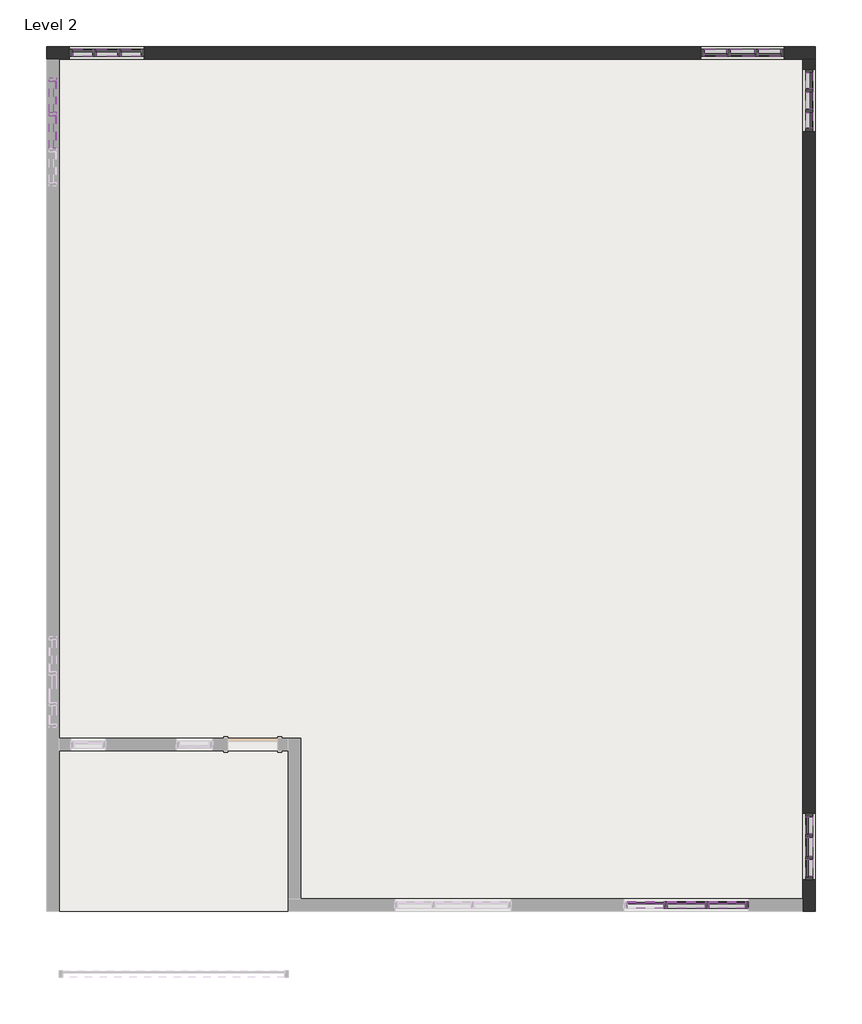
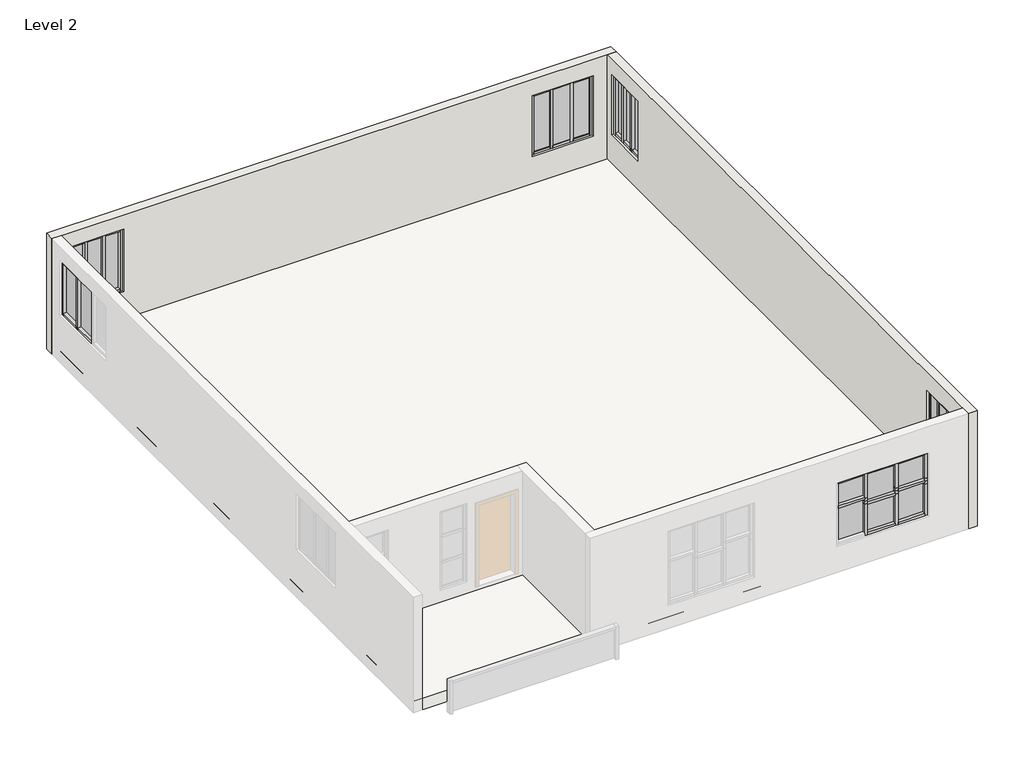
# One storey, part 2 of 2: 65 members, 20 plates, 2 walls, 1 roof.
"""IFC4 building model written with IfcOpenShell, lengths in millimetres."""

from ifc_helpers import new_model, si_unit, frame, origin, place, context, project, spatial, polyline, outline, extrude, faceted_brep, transform, mapped, element, save
from components import member_dc106669, member_bc7dbe04, member_b955a9e9, member_c33c434a, member_5ad95953, member_ff1b7d8f, member_c71c3647, member_d485efb4, member_6c34f49c, member_3060f3e2, member_dfbe775a, member_db0015e1, member_7096a90e, member_843225dc, member_fad113ab, member_ea29af33, member_6f432376, member_04a79ac1, member_a400357f, member_b1615173, member_de6f3820, member_f53dc333, member_00d00b53, member_c7c5a8a0, member_d6240b74, member_2ee2964b, member_655cfd9b, member_3d7cb871, member_3cc62806, member_2ad165f7, system_panel_glazed_811a1c5c, system_panel_glazed_f11b7ff6, system_panel_glazed_c33e710a, system_panel_glazed_37470fb4, system_panel_glazed_1aec69dd, system_panel_glazed_f4403250, system_panel_glazed_a7448bf8, system_panel_glazed_01fedee4, system_panel_glazed_02e859a2, system_panel_glazed_cd5540fc, system_panel_glazed_1b56a55a, system_panel_glazed_4819e94b, system_panel_glazed_cfa4a589, system_panel_glazed_093ce7df, system_panel_glazed_0a1fe405, system_panel_glazed_81358e4c

model = new_model("IFC4")

# Units and contexts
model_context = context("Model", 3, world=origin())
ifc_project = project(units=[si_unit("LENGTHUNIT", "METRE", prefix="MILLI")], contexts=[model_context])

# Site, building, storey
site = spatial("IfcSite", under=ifc_project)
building = spatial("IfcBuilding", under=site)
storey = spatial("IfcBuildingStorey", under=building, Name="Level 2", Elevation=3048.0)

# Members
placement = place(None, origin())
member_shape = member_dc106669(model_context)
element("IfcMember", 1, ObjectType="Rectangular Mullion : 2.5\" x 5\" rectangular", at=placement, inside=storey, context=model_context, shape_type="MappedRepresentation", body=[
    mapped(member_shape, transform((-8840.6597681, 1450.4660078, 5670.8139768), x_axis=(0.0, 0.0, 1.0), y_axis=(0.0, 1.0, 0.0), z_axis=(-1.0, 0.0, 0.0))),
])
element("IfcMember", 2, ObjectType="Rectangular Mullion : 2.5\" x 5\" rectangular", at=placement, inside=storey, context=model_context, shape_type="MappedRepresentation", body=[
    mapped(member_shape, transform((-9824.9097681, 1450.4660078, 5670.8139768), x_axis=(0.0, 0.0, 1.0), y_axis=(0.0, 1.0, 0.0), z_axis=(-1.0, 0.0, 0.0))),
])
member_2_shape = member_bc7dbe04(model_context)
element("IfcMember", 3, ObjectType="Rectangular Mullion : 2.5\" x 5\" rectangular", at=placement, inside=storey, context=model_context, shape_type="MappedRepresentation", body=[
    mapped(member_2_shape, transform((-9348.6597681, 1450.4660078, 5670.8139768), x_axis=(0.0, 0.0, 1.0), y_axis=(0.0, 1.0, 0.0), z_axis=(-1.0, 0.0, 0.0))),
])
element("IfcMember", 4, ObjectType="Rectangular Mullion : 2.5\" x 5\" rectangular", at=placement, inside=storey, context=model_context, shape_type="MappedRepresentation", body=[
    mapped(member_2_shape, transform((-8904.1597681, 1450.4660078, 4071.2518782), x_axis=(0.0, 0.0, -1.0), y_axis=(0.0, 1.0, 0.0), z_axis=(1.0, 0.0, 0.0))),
])
element("IfcMember", 5, ObjectType="Rectangular Mullion : 2.5\" x 5\" rectangular", at=placement, inside=storey, context=model_context, shape_type="MappedRepresentation", body=[
    mapped(member_shape, transform((-9412.1597681, 1450.4660078, 4071.2518782), x_axis=(0.0, 0.0, -1.0), y_axis=(0.0, 1.0, 0.0), z_axis=(1.0, 0.0, 0.0))),
])
element("IfcMember", 6, ObjectType="Rectangular Mullion : 2.5\" x 5\" rectangular", at=placement, inside=storey, context=model_context, shape_type="MappedRepresentation", body=[
    mapped(member_shape, transform((-8427.9097681, 1450.4660078, 4071.2518782), x_axis=(0.0, 0.0, -1.0), y_axis=(0.0, 1.0, 0.0), z_axis=(1.0, 0.0, 0.0))),
])
member_3_shape = member_b955a9e9(model_context)
element("IfcMember", 7, ObjectType="Rectangular Mullion : 2.5\" x 5\" rectangular", at=placement, inside=storey, context=model_context, shape_type="MappedRepresentation", body=[
    mapped(member_3_shape, transform((-9805.8597681, -14132.4339922, 5397.3589008), x_axis=(0.0, 0.0, 1.0), y_axis=(0.0, -1.0, 0.0), z_axis=(1.0, 0.0, 0.0))),
])
member_4_shape = member_c33c434a(model_context)
element("IfcMember", 8, ObjectType="Rectangular Mullion : 2.5\" x 5\" rectangular", at=placement, inside=storey, context=model_context, shape_type="MappedRepresentation", body=[
    mapped(member_4_shape, transform((-10567.8597681, -14132.4339922, 5397.3589008), x_axis=(0.0, 0.0, 1.0), y_axis=(0.0, -1.0, 0.0), z_axis=(1.0, 0.0, 0.0))),
])
element("IfcMember", 9, ObjectType="Rectangular Mullion : 2.5\" x 5\" rectangular", at=placement, inside=storey, context=model_context, shape_type="MappedRepresentation", body=[
    mapped(member_4_shape, transform((-9075.6097681, -14132.4339922, 5397.3589008), x_axis=(0.0, 0.0, 1.0), y_axis=(0.0, -1.0, 0.0), z_axis=(1.0, 0.0, 0.0))),
])
element("IfcMember", 10, ObjectType="Rectangular Mullion : 2.5\" x 5\" rectangular", at=placement, inside=storey, context=model_context, shape_type="MappedRepresentation", body=[
    mapped(member_4_shape, transform((-9742.3597681, -14132.4339922, 3732.481147), x_axis=(0.0, 0.0, -1.0), y_axis=(0.0, -1.0, 0.0), z_axis=(-1.0, 0.0, 0.0))),
])
element("IfcMember", 11, ObjectType="Rectangular Mullion : 2.5\" x 5\" rectangular", at=placement, inside=storey, context=model_context, shape_type="MappedRepresentation", body=[
    mapped(member_3_shape, transform((-10504.3597681, -14132.4339922, 3732.481147), x_axis=(0.0, 0.0, -1.0), y_axis=(0.0, -1.0, 0.0), z_axis=(-1.0, 0.0, 0.0))),
])
member_5_shape = member_5ad95953(model_context)
element("IfcMember", 12, ObjectType="Rectangular Mullion : 2.5\" x 5\" rectangular", at=placement, inside=storey, context=model_context, shape_type="MappedRepresentation", body=[
    mapped(member_5_shape, transform((-7907.2097681, -13300.5839922, 5612.7165878), x_axis=(0.0, 0.0, 1.0), y_axis=(1.0, 0.0, 0.0), z_axis=(0.0, 1.0, 0.0))),
])
element("IfcMember", 13, ObjectType="Rectangular Mullion : 2.5\" x 5\" rectangular", at=placement, inside=storey, context=model_context, shape_type="MappedRepresentation", body=[
    mapped(member_5_shape, transform((-7907.2097681, -12519.5339922, 5612.7165878), x_axis=(0.0, 0.0, 1.0), y_axis=(1.0, 0.0, 0.0), z_axis=(0.0, 1.0, 0.0))),
])
member_6_shape = member_ff1b7d8f(model_context)
element("IfcMember", 14, ObjectType="Rectangular Mullion : 2.5\" x 5\" rectangular", at=placement, inside=storey, context=model_context, shape_type="MappedRepresentation", body=[
    mapped(member_6_shape, transform((-7907.2097681, -12894.1839922, 5612.7165878), x_axis=(0.0, 0.0, 1.0), y_axis=(1.0, 0.0, 0.0), z_axis=(0.0, 1.0, 0.0))),
])
member_7_shape = member_c71c3647(model_context)
element("IfcMember", 15, ObjectType="Rectangular Mullion : 2.5\" x 5\" rectangular", at=placement, inside=storey, context=model_context, shape_type="MappedRepresentation", body=[
    mapped(member_7_shape, transform((-7907.2097681, -12862.4339922, 4117.147182), x_axis=(0.0, 1.0, 0.0), y_axis=(1.0, 0.0, 0.0), z_axis=(0.0, 0.0, -1.0))),
])
element("IfcMember", 16, ObjectType="Rectangular Mullion : 2.5\" x 5\" rectangular", at=placement, inside=storey, context=model_context, shape_type="MappedRepresentation", body=[
    mapped(member_7_shape, transform((-7907.2097681, -13268.8339922, 4117.147182), x_axis=(0.0, 1.0, 0.0), y_axis=(1.0, 0.0, 0.0), z_axis=(0.0, 0.0, -1.0))),
])
element("IfcMember", 17, ObjectType="Rectangular Mullion : 2.5\" x 5\" rectangular", at=placement, inside=storey, context=model_context, shape_type="MappedRepresentation", body=[
    mapped(member_5_shape, transform((-7907.2097681, -12830.6839922, 4117.147182), x_axis=(0.0, 0.0, -1.0), y_axis=(1.0, 0.0, 0.0), z_axis=(0.0, -1.0, 0.0))),
])
element("IfcMember", 18, ObjectType="Rectangular Mullion : 2.5\" x 5\" rectangular", at=placement, inside=storey, context=model_context, shape_type="MappedRepresentation", body=[
    mapped(member_5_shape, transform((-7907.2097681, -13611.7339922, 4117.147182), x_axis=(0.0, 0.0, -1.0), y_axis=(1.0, 0.0, 0.0), z_axis=(0.0, -1.0, 0.0))),
])
element("IfcMember", 19, ObjectType="Rectangular Mullion : 2.5\" x 5\" rectangular", at=placement, inside=storey, context=model_context, shape_type="MappedRepresentation", body=[
    mapped(member_6_shape, transform((-7907.2097681, -13237.0839922, 4117.147182), x_axis=(0.0, 0.0, -1.0), y_axis=(1.0, 0.0, 0.0), z_axis=(0.0, -1.0, 0.0))),
])
member_8_shape = member_d485efb4(model_context)
element("IfcMember", 20, ObjectType="Rectangular Mullion : 2.5\" x 5\" rectangular", at=placement, inside=storey, context=model_context, shape_type="MappedRepresentation", body=[
    mapped(member_8_shape, transform((-7907.2097681, -12456.0339922, 4117.147182), x_axis=(0.0, 1.0, 0.0), y_axis=(1.0, 0.0, 0.0), z_axis=(0.0, 0.0, -1.0))),
])
element("IfcMember", 21, ObjectType="Rectangular Mullion : 2.5\" x 5\" rectangular", at=placement, inside=storey, context=model_context, shape_type="MappedRepresentation", body=[
    mapped(member_8_shape, transform((-7907.2097681, -13675.2339922, 5612.7165878), x_axis=(0.0, -1.0, 0.0), y_axis=(1.0, 0.0, 0.0), z_axis=(0.0, 0.0, 1.0))),
])
member_9_shape = member_6c34f49c(model_context)
element("IfcMember", 22, ObjectType="Rectangular Mullion : 2.5\" x 5\" rectangular", at=placement, inside=storey, context=model_context, shape_type="MappedRepresentation", body=[
    mapped(member_9_shape, transform((-7907.2097681, 796.4160078, 5681.6996077), x_axis=(0.0, 0.0, 1.0), y_axis=(-1.0, 0.0, 0.0), z_axis=(0.0, -1.0, 0.0))),
])
element("IfcMember", 23, ObjectType="Rectangular Mullion : 2.5\" x 5\" rectangular", at=placement, inside=storey, context=model_context, shape_type="MappedRepresentation", body=[
    mapped(member_9_shape, transform((-7907.2097681, 66.1660078, 5681.6996077), x_axis=(0.0, 0.0, 1.0), y_axis=(-1.0, 0.0, 0.0), z_axis=(0.0, -1.0, 0.0))),
])
member_10_shape = member_3060f3e2(model_context)
element("IfcMember", 24, ObjectType="Rectangular Mullion : 2.5\" x 5\" rectangular", at=placement, inside=storey, context=model_context, shape_type="MappedRepresentation", body=[
    mapped(member_10_shape, transform((-7907.2097681, 415.4160078, 5681.6996077), x_axis=(0.0, 0.0, 1.0), y_axis=(-1.0, 0.0, 0.0), z_axis=(0.0, -1.0, 0.0))),
])
member_11_shape = member_dfbe775a(model_context)
element("IfcMember", 25, ObjectType="Rectangular Mullion : 2.5\" x 5\" rectangular", at=placement, inside=storey, context=model_context, shape_type="MappedRepresentation", body=[
    mapped(member_11_shape, transform((-7907.2097681, 383.6660078, 4107.4707945), x_axis=(0.0, -1.0, 0.0), y_axis=(-1.0, 0.0, 0.0), z_axis=(0.0, 0.0, -1.0))),
])
element("IfcMember", 26, ObjectType="Rectangular Mullion : 2.5\" x 5\" rectangular", at=placement, inside=storey, context=model_context, shape_type="MappedRepresentation", body=[
    mapped(member_11_shape, transform((-7907.2097681, 764.6660078, 4107.4707945), x_axis=(0.0, -1.0, 0.0), y_axis=(-1.0, 0.0, 0.0), z_axis=(0.0, 0.0, -1.0))),
])
element("IfcMember", 27, ObjectType="Rectangular Mullion : 2.5\" x 5\" rectangular", at=placement, inside=storey, context=model_context, shape_type="MappedRepresentation", body=[
    mapped(member_10_shape, transform((-7907.2097681, 732.9160078, 4107.4707945), x_axis=(0.0, 0.0, -1.0), y_axis=(-1.0, 0.0, 0.0), z_axis=(0.0, 1.0, 0.0))),
])
element("IfcMember", 28, ObjectType="Rectangular Mullion : 2.5\" x 5\" rectangular", at=placement, inside=storey, context=model_context, shape_type="MappedRepresentation", body=[
    mapped(member_9_shape, transform((-7907.2097681, 351.9160078, 4107.4707945), x_axis=(0.0, 0.0, -1.0), y_axis=(-1.0, 0.0, 0.0), z_axis=(0.0, 1.0, 0.0))),
])
element("IfcMember", 29, ObjectType="Rectangular Mullion : 2.5\" x 5\" rectangular", at=placement, inside=storey, context=model_context, shape_type="MappedRepresentation", body=[
    mapped(member_9_shape, transform((-7907.2097681, 1082.1660078, 4107.4707945), x_axis=(0.0, 0.0, -1.0), y_axis=(-1.0, 0.0, 0.0), z_axis=(0.0, 1.0, 0.0))),
])
member_12_shape = member_db0015e1(model_context)
element("IfcMember", 30, ObjectType="Rectangular Mullion : 2.5\" x 5\" rectangular", at=placement, inside=storey, context=model_context, shape_type="MappedRepresentation", body=[
    mapped(member_12_shape, transform((-7907.2097681, 1145.6660078, 5681.6996077), x_axis=(0.0, 1.0, 0.0), y_axis=(-1.0, 0.0, 0.0), z_axis=(0.0, 0.0, 1.0))),
])
element("IfcMember", 31, ObjectType="Rectangular Mullion : 2.5\" x 5\" rectangular", at=placement, inside=storey, context=model_context, shape_type="MappedRepresentation", body=[
    mapped(member_12_shape, transform((-7907.2097681, 2.6660078, 4107.4707945), x_axis=(0.0, -1.0, 0.0), y_axis=(-1.0, 0.0, 0.0), z_axis=(0.0, 0.0, -1.0))),
])
member_13_shape = member_7096a90e(model_context)
element("IfcMember", 32, ObjectType="Rectangular Mullion : 2.5\" x 5\" rectangular", at=placement, inside=storey, context=model_context, shape_type="MappedRepresentation", body=[
    mapped(member_13_shape, transform((-20550.0597681, 1450.4660078, 5713.3390555), x_axis=(0.0, 0.0, 1.0), y_axis=(0.0, -1.0, 0.0), z_axis=(1.0, 0.0, 0.0))),
])
member_14_shape = member_843225dc(model_context)
element("IfcMember", 33, ObjectType="Rectangular Mullion : 2.5\" x 5\" rectangular", at=placement, inside=storey, context=model_context, shape_type="MappedRepresentation", body=[
    mapped(member_14_shape, transform((-21007.2597681, 1450.4660078, 5713.3390555), x_axis=(0.0, 0.0, 1.0), y_axis=(0.0, -1.0, 0.0), z_axis=(1.0, 0.0, 0.0))),
])
element("IfcMember", 34, ObjectType="Rectangular Mullion : 2.5\" x 5\" rectangular", at=placement, inside=storey, context=model_context, shape_type="MappedRepresentation", body=[
    mapped(member_14_shape, transform((-20124.6097681, 1450.4660078, 5713.3390555), x_axis=(0.0, 0.0, 1.0), y_axis=(0.0, -1.0, 0.0), z_axis=(1.0, 0.0, 0.0))),
])
member_15_shape = member_fad113ab(model_context)
element("IfcMember", 35, ObjectType="Rectangular Mullion : 2.5\" x 5\" rectangular", at=placement, inside=storey, context=model_context, shape_type="MappedRepresentation", body=[
    mapped(member_15_shape, transform((-20518.3097681, 1450.4660078, 4066.3851852), x_axis=(1.0, 0.0, 0.0), y_axis=(0.0, -1.0, 0.0), z_axis=(0.0, 0.0, -1.0))),
])
element("IfcMember", 36, ObjectType="Rectangular Mullion : 2.5\" x 5\" rectangular", at=placement, inside=storey, context=model_context, shape_type="MappedRepresentation", body=[
    mapped(member_15_shape, transform((-20975.5097681, 1450.4660078, 4066.3851852), x_axis=(1.0, 0.0, 0.0), y_axis=(0.0, -1.0, 0.0), z_axis=(0.0, 0.0, -1.0))),
])
element("IfcMember", 37, ObjectType="Rectangular Mullion : 2.5\" x 5\" rectangular", at=placement, inside=storey, context=model_context, shape_type="MappedRepresentation", body=[
    mapped(member_13_shape, transform((-20943.7597681, 1450.4660078, 4066.3851852), x_axis=(0.0, 0.0, -1.0), y_axis=(0.0, -1.0, 0.0), z_axis=(-1.0, 0.0, 0.0))),
])
element("IfcMember", 38, ObjectType="Rectangular Mullion : 2.5\" x 5\" rectangular", at=placement, inside=storey, context=model_context, shape_type="MappedRepresentation", body=[
    mapped(member_14_shape, transform((-20486.5597681, 1450.4660078, 4066.3851852), x_axis=(0.0, 0.0, -1.0), y_axis=(0.0, -1.0, 0.0), z_axis=(-1.0, 0.0, 0.0))),
])
element("IfcMember", 39, ObjectType="Rectangular Mullion : 2.5\" x 5\" rectangular", at=placement, inside=storey, context=model_context, shape_type="MappedRepresentation", body=[
    mapped(member_14_shape, transform((-21369.2097681, 1450.4660078, 4066.3851852), x_axis=(0.0, 0.0, -1.0), y_axis=(0.0, -1.0, 0.0), z_axis=(-1.0, 0.0, 0.0))),
])
member_16_shape = member_ea29af33(model_context)
element("IfcMember", 40, ObjectType="Rectangular Mullion : 2.5\" x 5\" rectangular", at=placement, inside=storey, context=model_context, shape_type="MappedRepresentation", body=[
    mapped(member_16_shape, transform((-21432.7097681, 1450.4660078, 5713.3390555), x_axis=(-1.0, 0.0, 0.0), y_axis=(0.0, -1.0, 0.0), z_axis=(0.0, 0.0, 1.0))),
])
element("IfcMember", 41, ObjectType="Rectangular Mullion : 2.5\" x 5\" rectangular", at=placement, inside=storey, context=model_context, shape_type="MappedRepresentation", body=[
    mapped(member_16_shape, transform((-20061.1097681, 1450.4660078, 4066.3851852), x_axis=(1.0, 0.0, 0.0), y_axis=(0.0, -1.0, 0.0), z_axis=(0.0, 0.0, -1.0))),
])
member_17_shape = member_6f432376(model_context)
element("IfcMember", 42, ObjectType="Rectangular Mullion : 2.5\" x 5\" rectangular", at=placement, inside=storey, context=model_context, shape_type="MappedRepresentation", body=[
    mapped(member_17_shape, transform((-21737.5097681, 364.6160078, 5718.9037492), x_axis=(0.0, 0.0, 1.0), y_axis=(-1.0, 0.0, 0.0), z_axis=(0.0, -1.0, 0.0))),
])
member_18_shape = member_04a79ac1(model_context)
element("IfcMember", 43, ObjectType="Rectangular Mullion : 2.5\" x 5\" rectangular", at=placement, inside=storey, context=model_context, shape_type="MappedRepresentation", body=[
    mapped(member_18_shape, transform((-21737.5097681, 332.8660078, 4287.8866443), x_axis=(0.0, -1.0, 0.0), y_axis=(-1.0, 0.0, 0.0), z_axis=(0.0, 0.0, -1.0))),
])
element("IfcMember", 44, ObjectType="Rectangular Mullion : 2.5\" x 5\" rectangular", at=placement, inside=storey, context=model_context, shape_type="MappedRepresentation", body=[
    mapped(member_17_shape, transform((-21737.5097681, 929.7660078, 4287.8866443), x_axis=(0.0, 0.0, -1.0), y_axis=(-1.0, 0.0, 0.0), z_axis=(0.0, 1.0, 0.0))),
])
member_19_shape = member_a400357f(model_context)
element("IfcMember", 45, ObjectType="Rectangular Mullion : 2.5\" x 5\" rectangular", at=placement, inside=storey, context=model_context, shape_type="MappedRepresentation", body=[
    mapped(member_19_shape, transform((-21737.5097681, 301.1160078, 4287.8866443), x_axis=(0.0, 0.0, -1.0), y_axis=(-1.0, 0.0, 0.0), z_axis=(0.0, 1.0, 0.0))),
])
member_20_shape = member_b1615173(model_context)
element("IfcMember", 46, ObjectType="Rectangular Mullion : 2.5\" x 5\" rectangular", at=placement, inside=storey, context=model_context, shape_type="MappedRepresentation", body=[
    mapped(member_20_shape, transform((-21737.5097681, 993.2660078, 5718.9037492), x_axis=(0.0, 1.0, 0.0), y_axis=(-1.0, 0.0, 0.0), z_axis=(0.0, 0.0, 1.0))),
])
member_21_shape = member_de6f3820(model_context)
element("IfcMember", 47, ObjectType="Rectangular Mullion : 2.5\" x 5\" rectangular", at=placement, inside=storey, context=model_context, shape_type="MappedRepresentation", body=[
    mapped(member_21_shape, transform((-9380.4097681, 1450.4660078, 4071.2518782), x_axis=(-1.0, 0.0, 0.0), y_axis=(0.0, 1.0, 0.0), z_axis=(0.0, 0.0, -1.0))),
])
element("IfcMember", 48, ObjectType="Rectangular Mullion : 2.5\" x 5\" rectangular", at=placement, inside=storey, context=model_context, shape_type="MappedRepresentation", body=[
    mapped(member_21_shape, transform((-8872.4097681, 1450.4660078, 4071.2518782), x_axis=(-1.0, 0.0, 0.0), y_axis=(0.0, 1.0, 0.0), z_axis=(0.0, 0.0, -1.0))),
])
member_22_shape = member_f53dc333(model_context)
element("IfcMember", 49, ObjectType="Rectangular Mullion : 2.5\" x 5\" rectangular", at=placement, inside=storey, context=model_context, shape_type="MappedRepresentation", body=[
    mapped(member_22_shape, transform((-9888.4097681, 1450.4660078, 4071.2518782), x_axis=(-1.0, 0.0, 0.0), y_axis=(0.0, 1.0, 0.0), z_axis=(0.0, 0.0, -1.0))),
])
element("IfcMember", 50, ObjectType="Rectangular Mullion : 2.5\" x 5\" rectangular", at=placement, inside=storey, context=model_context, shape_type="MappedRepresentation", body=[
    mapped(member_22_shape, transform((-8364.4097681, 1450.4660078, 5670.8139768), x_axis=(1.0, 0.0, 0.0), y_axis=(0.0, 1.0, 0.0), z_axis=(0.0, 0.0, 1.0))),
])
member_23_shape = member_00d00b53(model_context)
element("IfcMember", 51, ObjectType="Rectangular Mullion : 2.5\" x 5\" rectangular", at=placement, inside=storey, context=model_context, shape_type="MappedRepresentation", body=[
    mapped(member_23_shape, transform((-9774.1097681, -14132.4339922, 4641.1200239), x_axis=(1.0, 0.0, 0.0), y_axis=(0.0, -1.0, 0.0), z_axis=(0.0, 0.0, -1.0))),
])
element("IfcMember", 52, ObjectType="Rectangular Mullion : 2.5\" x 5\" rectangular", at=placement, inside=storey, context=model_context, shape_type="MappedRepresentation", body=[
    mapped(member_23_shape, transform((-10536.1097681, -14132.4339922, 4564.9200239), x_axis=(1.0, 0.0, 0.0), y_axis=(0.0, -1.0, 0.0), z_axis=(0.0, 0.0, -1.0))),
])
element("IfcMember", 53, ObjectType="Rectangular Mullion : 2.5\" x 5\" rectangular", at=placement, inside=storey, context=model_context, shape_type="MappedRepresentation", body=[
    mapped(member_23_shape, transform((-9774.1097681, -14132.4339922, 4564.9200239), x_axis=(1.0, 0.0, 0.0), y_axis=(0.0, -1.0, 0.0), z_axis=(0.0, 0.0, -1.0))),
])
member_24_shape = member_c7c5a8a0(model_context)
element("IfcMember", 54, ObjectType="Rectangular Mullion : 2.5\" x 5\" rectangular", at=placement, inside=storey, context=model_context, shape_type="MappedRepresentation", body=[
    mapped(member_24_shape, transform((-9805.8597681, -14132.4339922, 4564.9200239), x_axis=(0.0, 0.0, 1.0), y_axis=(0.0, -1.0, 0.0), z_axis=(1.0, 0.0, 0.0))),
])
element("IfcMember", 55, ObjectType="Rectangular Mullion : 2.5\" x 5\" rectangular", at=placement, inside=storey, context=model_context, shape_type="MappedRepresentation", body=[
    mapped(member_23_shape, transform((-10536.1097681, -14132.4339922, 4641.1200239), x_axis=(1.0, 0.0, 0.0), y_axis=(0.0, -1.0, 0.0), z_axis=(0.0, 0.0, -1.0))),
])
member_25_shape = member_d6240b74(model_context)
element("IfcMember", 56, ObjectType="Rectangular Mullion : 2.5\" x 5\" rectangular", at=placement, inside=storey, context=model_context, shape_type="MappedRepresentation", body=[
    mapped(member_25_shape, transform((-9774.1097681, -14132.4339922, 4717.3200239), x_axis=(1.0, 0.0, 0.0), y_axis=(0.0, -1.0, 0.0), z_axis=(0.0, 0.0, -1.0))),
])
element("IfcMember", 57, ObjectType="Rectangular Mullion : 2.5\" x 5\" rectangular", at=placement, inside=storey, context=model_context, shape_type="MappedRepresentation", body=[
    mapped(member_25_shape, transform((-10536.1097681, -14132.4339922, 4717.3200239), x_axis=(1.0, 0.0, 0.0), y_axis=(0.0, -1.0, 0.0), z_axis=(0.0, 0.0, -1.0))),
])
member_26_shape = member_2ee2964b(model_context)
element("IfcMember", 58, ObjectType="Rectangular Mullion : 2.5\" x 5\" rectangular", at=placement, inside=storey, context=model_context, shape_type="MappedRepresentation", body=[
    mapped(member_26_shape, transform((-10567.8597681, -14132.4339922, 4717.3200239), x_axis=(0.0, 0.0, 1.0), y_axis=(0.0, -1.0, 0.0), z_axis=(1.0, 0.0, 0.0))),
])
element("IfcMember", 59, ObjectType="Rectangular Mullion : 2.5\" x 5\" rectangular", at=placement, inside=storey, context=model_context, shape_type="MappedRepresentation", body=[
    mapped(member_26_shape, transform((-9075.6097681, -14132.4339922, 4641.1200239), x_axis=(0.0, 0.0, 1.0), y_axis=(0.0, -1.0, 0.0), z_axis=(1.0, 0.0, 0.0))),
])
member_27_shape = member_655cfd9b(model_context)
element("IfcMember", 60, ObjectType="Rectangular Mullion : 2.5\" x 5\" rectangular", at=placement, inside=storey, context=model_context, shape_type="MappedRepresentation", body=[
    mapped(member_27_shape, transform((-9774.1097681, -14132.4339922, 3732.481147), x_axis=(1.0, 0.0, 0.0), y_axis=(0.0, -1.0, 0.0), z_axis=(0.0, 0.0, -1.0))),
])
element("IfcMember", 61, ObjectType="Rectangular Mullion : 2.5\" x 5\" rectangular", at=placement, inside=storey, context=model_context, shape_type="MappedRepresentation", body=[
    mapped(member_27_shape, transform((-10536.1097681, -14132.4339922, 3732.481147), x_axis=(1.0, 0.0, 0.0), y_axis=(0.0, -1.0, 0.0), z_axis=(0.0, 0.0, -1.0))),
])
member_28_shape = member_3d7cb871(model_context)
element("IfcMember", 62, ObjectType="Rectangular Mullion : 2.5\" x 5\" rectangular", at=placement, inside=storey, context=model_context, shape_type="MappedRepresentation", body=[
    mapped(member_28_shape, transform((-9012.1097681, -14132.4339922, 4641.1200239), x_axis=(1.0, 0.0, 0.0), y_axis=(0.0, -1.0, 0.0), z_axis=(0.0, 0.0, -1.0))),
])
member_29_shape = member_3cc62806(model_context)
element("IfcMember", 63, ObjectType="Rectangular Mullion : 2.5\" x 5\" rectangular", at=placement, inside=storey, context=model_context, shape_type="MappedRepresentation", body=[
    mapped(member_29_shape, transform((-9012.1097681, -14132.4339922, 4717.3200239), x_axis=(1.0, 0.0, 0.0), y_axis=(0.0, -1.0, 0.0), z_axis=(0.0, 0.0, -1.0))),
])
element("IfcMember", 64, ObjectType="Rectangular Mullion : 2.5\" x 5\" rectangular", at=placement, inside=storey, context=model_context, shape_type="MappedRepresentation", body=[
    mapped(member_28_shape, transform((-9012.1097681, -14132.4339922, 4564.9200239), x_axis=(1.0, 0.0, 0.0), y_axis=(0.0, -1.0, 0.0), z_axis=(0.0, 0.0, -1.0))),
])
member_30_shape = member_2ad165f7(model_context)
element("IfcMember", 65, ObjectType="Rectangular Mullion : 2.5\" x 5\" rectangular", at=placement, inside=storey, context=model_context, shape_type="MappedRepresentation", body=[
    mapped(member_30_shape, transform((-9012.1097681, -14132.4339922, 3732.481147), x_axis=(1.0, 0.0, 0.0), y_axis=(0.0, -1.0, 0.0), z_axis=(0.0, 0.0, -1.0))),
])

# Plates
system_panel_glazed_shape = system_panel_glazed_811a1c5c(model_context)
element("IfcPlate", 66, ObjectType="System Panel : Glazed", at=placement, inside=storey, context=model_context, shape_type="MappedRepresentation", body=[
    mapped(system_panel_glazed_shape, transform((-7907.2097681, -13456.1589922, 4180.647182), x_axis=(0.0, 1.0, 0.0), y_axis=(-1.0, 0.0, 0.0), z_axis=(0.0, 0.0, 1.0))),
])
element("IfcPlate", 67, ObjectType="System Panel : Glazed", at=placement, inside=storey, context=model_context, shape_type="MappedRepresentation", body=[
    mapped(system_panel_glazed_shape, transform((-7907.2097681, -12675.1089922, 4180.647182), x_axis=(0.0, 1.0, 0.0), y_axis=(-1.0, 0.0, 0.0), z_axis=(0.0, 0.0, 1.0))),
])
system_panel_glazed_2_shape = system_panel_glazed_f11b7ff6(model_context)
element("IfcPlate", 68, ObjectType="System Panel : Glazed", at=placement, inside=storey, context=model_context, shape_type="MappedRepresentation", body=[
    mapped(system_panel_glazed_2_shape, transform((-7907.2097681, -13065.6339922, 4180.647182), x_axis=(0.0, 1.0, 0.0), y_axis=(-1.0, 0.0, 0.0), z_axis=(0.0, 0.0, 1.0))),
])
system_panel_glazed_3_shape = system_panel_glazed_c33e710a(model_context)
element("IfcPlate", 69, ObjectType="System Panel : Glazed", at=placement, inside=storey, context=model_context, shape_type="MappedRepresentation", body=[
    mapped(system_panel_glazed_3_shape, transform((-7907.2097681, 939.2910078, 4170.9707945), x_axis=(0.0, -1.0, 0.0), y_axis=(1.0, 0.0, 0.0), z_axis=(0.0, 0.0, 1.0))),
])
element("IfcPlate", 70, ObjectType="System Panel : Glazed", at=placement, inside=storey, context=model_context, shape_type="MappedRepresentation", body=[
    mapped(system_panel_glazed_3_shape, transform((-7907.2097681, 209.0410078, 4170.9707945), x_axis=(0.0, -1.0, 0.0), y_axis=(1.0, 0.0, 0.0), z_axis=(0.0, 0.0, 1.0))),
])
system_panel_glazed_4_shape = system_panel_glazed_37470fb4(model_context)
element("IfcPlate", 71, ObjectType="System Panel : Glazed", at=placement, inside=storey, context=model_context, shape_type="MappedRepresentation", body=[
    mapped(system_panel_glazed_4_shape, transform((-7907.2097681, 574.1660078, 4170.9707945), x_axis=(0.0, -1.0, 0.0), y_axis=(1.0, 0.0, 0.0), z_axis=(0.0, 0.0, 1.0))),
])
system_panel_glazed_5_shape = system_panel_glazed_1aec69dd(model_context)
element("IfcPlate", 72, ObjectType="System Panel : Glazed", at=placement, inside=storey, context=model_context, shape_type="MappedRepresentation", body=[
    mapped(system_panel_glazed_5_shape, transform((-21188.2347681, 1450.4660078, 4129.8851852), x_axis=(1.0, 0.0, 0.0), y_axis=(0.0, 1.0, 0.0), z_axis=(0.0, 0.0, 1.0))),
])
element("IfcPlate", 73, ObjectType="System Panel : Glazed", at=placement, inside=storey, context=model_context, shape_type="MappedRepresentation", body=[
    mapped(system_panel_glazed_5_shape, transform((-20305.5847681, 1450.4660078, 4129.8851852), x_axis=(1.0, 0.0, 0.0), y_axis=(0.0, 1.0, 0.0), z_axis=(0.0, 0.0, 1.0))),
])
system_panel_glazed_6_shape = system_panel_glazed_f4403250(model_context)
element("IfcPlate", 74, ObjectType="System Panel : Glazed", at=placement, inside=storey, context=model_context, shape_type="MappedRepresentation", body=[
    mapped(system_panel_glazed_6_shape, transform((-20746.9097681, 1450.4660078, 4129.8851852), x_axis=(1.0, 0.0, 0.0), y_axis=(0.0, 1.0, 0.0), z_axis=(0.0, 0.0, 1.0))),
])
system_panel_glazed_7_shape = system_panel_glazed_a7448bf8(model_context)
element("IfcPlate", 75, ObjectType="System Panel : Glazed", at=placement, inside=storey, context=model_context, shape_type="MappedRepresentation", body=[
    mapped(system_panel_glazed_7_shape, transform((-21737.5097681, 647.1910078, 4351.3866443), x_axis=(0.0, -1.0, 0.0), y_axis=(1.0, 0.0, 0.0), z_axis=(0.0, 0.0, 1.0))),
])
system_panel_glazed_8_shape = system_panel_glazed_01fedee4(model_context)
element("IfcPlate", 76, ObjectType="System Panel : Glazed", at=placement, inside=storey, context=model_context, shape_type="MappedRepresentation", body=[
    mapped(system_panel_glazed_8_shape, transform((-21737.5097681, 2.6660078, 4351.3866443), x_axis=(0.0, -1.0, 0.0), y_axis=(1.0, 0.0, 0.0), z_axis=(0.0, 0.0, 1.0))),
])
system_panel_glazed_9_shape = system_panel_glazed_02e859a2(model_context)
element("IfcPlate", 77, ObjectType="System Panel : Glazed", at=placement, inside=storey, context=model_context, shape_type="MappedRepresentation", body=[
    mapped(system_panel_glazed_9_shape, transform((-8634.2847681, 1450.4660078, 4134.7518782), x_axis=(-1.0, 0.0, 0.0), y_axis=(0.0, -1.0, 0.0), z_axis=(0.0, 0.0, 1.0))),
])
element("IfcPlate", 78, ObjectType="System Panel : Glazed", at=placement, inside=storey, context=model_context, shape_type="MappedRepresentation", body=[
    mapped(system_panel_glazed_9_shape, transform((-9618.5347681, 1450.4660078, 4134.7518782), x_axis=(-1.0, 0.0, 0.0), y_axis=(0.0, -1.0, 0.0), z_axis=(0.0, 0.0, 1.0))),
])
system_panel_glazed_10_shape = system_panel_glazed_cd5540fc(model_context)
element("IfcPlate", 79, ObjectType="System Panel : Glazed", at=placement, inside=storey, context=model_context, shape_type="MappedRepresentation", body=[
    mapped(system_panel_glazed_10_shape, transform((-9126.4097681, 1450.4660078, 4134.7518782), x_axis=(-1.0, 0.0, 0.0), y_axis=(0.0, -1.0, 0.0), z_axis=(0.0, 0.0, 1.0))),
])
system_panel_glazed_11_shape = system_panel_glazed_1b56a55a(model_context)
element("IfcPlate", 80, ObjectType="System Panel : Glazed", at=placement, inside=storey, context=model_context, shape_type="MappedRepresentation", body=[
    mapped(system_panel_glazed_11_shape, transform((-10155.1097681, -14132.4339922, 4596.6700239), x_axis=(1.0, 0.0, 0.0), y_axis=(0.0, 1.0, 0.0), z_axis=(0.0, 0.0, 1.0))),
])
system_panel_glazed_12_shape = system_panel_glazed_4819e94b(model_context)
element("IfcPlate", 81, ObjectType="System Panel : Glazed", at=placement, inside=storey, context=model_context, shape_type="MappedRepresentation", body=[
    mapped(system_panel_glazed_12_shape, transform((-10901.2347681, -14132.4339922, 4749.0700239), x_axis=(1.0, 0.0, 0.0), y_axis=(0.0, 1.0, 0.0), z_axis=(0.0, 0.0, 1.0))),
])
system_panel_glazed_13_shape = system_panel_glazed_cfa4a589(model_context)
element("IfcPlate", 82, ObjectType="System Panel : Glazed", at=placement, inside=storey, context=model_context, shape_type="MappedRepresentation", body=[
    mapped(system_panel_glazed_13_shape, transform((-10901.2347681, -14132.4339922, 3795.981147), x_axis=(1.0, 0.0, 0.0), y_axis=(0.0, 1.0, 0.0), z_axis=(0.0, 0.0, 1.0))),
])
system_panel_glazed_14_shape = system_panel_glazed_093ce7df(model_context)
element("IfcPlate", 83, ObjectType="System Panel : Glazed", at=placement, inside=storey, context=model_context, shape_type="MappedRepresentation", body=[
    mapped(system_panel_glazed_14_shape, transform((-10155.1097681, -14132.4339922, 3795.981147), x_axis=(1.0, 0.0, 0.0), y_axis=(0.0, 1.0, 0.0), z_axis=(0.0, 0.0, 1.0))),
])
system_panel_glazed_15_shape = system_panel_glazed_0a1fe405(model_context)
element("IfcPlate", 84, ObjectType="System Panel : Glazed", at=placement, inside=storey, context=model_context, shape_type="MappedRepresentation", body=[
    mapped(system_panel_glazed_15_shape, transform((-9408.9847681, -14132.4339922, 3795.981147), x_axis=(1.0, 0.0, 0.0), y_axis=(0.0, 1.0, 0.0), z_axis=(0.0, 0.0, 1.0))),
])
system_panel_glazed_16_shape = system_panel_glazed_81358e4c(model_context)
element("IfcPlate", 85, ObjectType="System Panel : Glazed", at=placement, inside=storey, context=model_context, shape_type="MappedRepresentation", body=[
    mapped(system_panel_glazed_16_shape, transform((-9408.9847681, -14132.4339922, 4672.8700239), x_axis=(1.0, 0.0, 0.0), y_axis=(0.0, 1.0, 0.0), z_axis=(0.0, 0.0, 1.0))),
])

# Roof
element("IfcRoof", 86, ObjectType="Generic - 12\"", at=placement, inside=storey, context=model_context, shape_type="SweptSolid", body=[
    extrude(outline(polyline([(-21851.8097681, 1564.7660078), (-7792.9097681, 1564.7660078), (-7792.9097681, -14246.7339922), (-21851.8097681, -14246.7339922), (-21851.8097681, 1564.7660078)])), frame((0.0, 0.0, 3048.0), z_axis=(0.0, 0.0, 1.0), x_axis=(1.0, 0.0, 0.0)), (0.0, 0.0, 1.0), 304.8),
])

# Walls
element("IfcWall", 87, ObjectType="9\"", at=placement, inside=storey, context=model_context, shape_type="Brep", body=[
    faceted_brep([(-21851.8097681, 1336.1660078, 3048.0), (-21623.2097681, 1336.1660078, 3048.0), (-8021.5097681, 1336.1660078, 3048.0), (-7792.9097681, 1336.1660078, 3048.0), (-7792.9097681, 1336.1660078, 6096.0), (-8021.5097681, 1336.1660078, 6096.0), (-21623.2097681, 1336.1660078, 6096.0), (-21851.8097681, 1336.1660078, 6096.0), (-21432.7097681, 1336.1660078, 4066.3851852), (-21432.7097681, 1336.1660078, 5713.3390555), (-20061.1097681, 1336.1660078, 5713.3390555), (-20061.1097681, 1336.1660078, 4066.3851852), (-8364.4097681, 1336.1660078, 5670.8139768), (-8364.4097681, 1336.1660078, 4071.2518782), (-9888.4097681, 1336.1660078, 4071.2518782), (-9888.4097681, 1336.1660078, 5670.8139768), (-7792.9097681, 1564.7660078, 3048.0), (-21851.8097681, 1564.7660078, 3048.0), (-21851.8097681, 1564.7660078, 6096.0), (-7792.9097681, 1564.7660078, 6096.0), (-21432.7097681, 1564.7660078, 5713.3390555), (-21432.7097681, 1564.7660078, 4066.3851852), (-20061.1097681, 1564.7660078, 4066.3851852), (-20061.1097681, 1564.7660078, 5713.3390555), (-8364.4097681, 1564.7660078, 4071.2518782), (-8364.4097681, 1564.7660078, 5670.8139768), (-9888.4097681, 1564.7660078, 5670.8139768), (-9888.4097681, 1564.7660078, 4071.2518782)], [[[0, 1, 2, 3, 4, 5, 6, 7], [8, 9, 10, 11], [12, 13, 14, 15]], [[16, 17, 18, 19], [20, 21, 22, 23], [24, 25, 26, 27]], [[3, 2, 1, 0, 17, 16]], [[7, 6, 5, 4, 19, 18]], [[4, 3, 16, 19]], [[0, 7, 18, 17]], [[20, 9, 8, 21]], [[9, 20, 23, 10]], [[10, 23, 22, 11]], [[21, 8, 11, 22]], [[24, 13, 12, 25]], [[25, 12, 15, 26]], [[26, 15, 14, 27]], [[13, 24, 27, 14]]]),
])
element("IfcWall", 88, ObjectType="9\"", at=placement, inside=storey, context=model_context, shape_type="Brep", body=[
    faceted_brep([(-8021.5097681, 1336.1660078, 3048.0), (-8021.5097681, -14018.1339922, 3048.0), (-8021.5097681, -14246.7339922, 3048.0), (-8021.5097681, -14246.7339922, 6096.0), (-8021.5097681, -14018.1339922, 6096.0), (-8021.5097681, 1336.1660078, 6096.0), (-8021.5097681, -13675.2339922, 5612.7165878), (-8021.5097681, -13675.2339922, 4117.147182), (-8021.5097681, -12456.0339922, 4117.147182), (-8021.5097681, -12456.0339922, 5612.7165878), (-8021.5097681, 1145.6660078, 4107.4707945), (-8021.5097681, 1145.6660078, 5681.6996077), (-8021.5097681, 2.6660078, 5681.6996077), (-8021.5097681, 2.6660078, 4107.4707945), (-7792.9097681, -14246.7339922, 3048.0), (-7792.9097681, 1336.1660078, 3048.0), (-7792.9097681, 1336.1660078, 6096.0), (-7792.9097681, -14246.7339922, 6096.0), (-7792.9097681, -13675.2339922, 4117.147182), (-7792.9097681, -13675.2339922, 5612.7165878), (-7792.9097681, -12456.0339922, 5612.7165878), (-7792.9097681, -12456.0339922, 4117.147182), (-7792.9097681, 1145.6660078, 5681.6996077), (-7792.9097681, 1145.6660078, 4107.4707945), (-7792.9097681, 2.6660078, 4107.4707945), (-7792.9097681, 2.6660078, 5681.6996077)], [[[0, 1, 2, 3, 4, 5], [6, 7, 8, 9], [10, 11, 12, 13]], [[14, 15, 16, 17], [18, 19, 20, 21], [22, 23, 24, 25]], [[2, 1, 0, 15, 14]], [[5, 4, 3, 17, 16]], [[0, 5, 16, 15]], [[3, 2, 14, 17]], [[18, 7, 6, 19]], [[19, 6, 9, 20]], [[20, 9, 8, 21]], [[7, 18, 21, 8]], [[22, 11, 10, 23]], [[11, 22, 25, 12]], [[12, 25, 24, 13]], [[23, 10, 13, 24]]]),
])

save(model, "model.ifc")

# Revit data of these elements
# Type "Rectangular Mullion : 2.5\" x 5\" rectangular"
#   built-in parameter 1007304 = 0.416667 (stored number, unit not read)
#   built-in parameter 1007301 = 0.104167 (stored number, unit not read)
#   built-in parameter 1007300 = 0.104167 (stored number, unit not read)
# Type "System Panel : Glazed"
#   Construction Type Id = "GSP4R"
#   Analytic Construction = "1/8 in Pilkington single glazing"
#   Visual Light Transmittance = 0.9
#   Solar Heat Gain Coefficient = 0.86
#   Heat Transfer Coefficient (U) = 1.18115 BTU/(h·ft²·°F)
#   Define Thermal Properties by = 1
# Type "Generic - 12\""
#   Assembly Code = "B1020"
#   Layers, outside or top first: 1' - 0" no material (function 1)
# Type "9\""
#   Assembly Code = "B2010"
#   Layers, outside or top first: 0' - 9" no material (function 1)
# Elements 1, 2, 3, 4, 5, 6, 7, 8, 9, 10, 11, 12, 13, 14, 15, 16, 17, 18, 19, 20, 21, 22, 23, 24, 25, 26, 27, 28, 29, 30, 31, 32, 33, 34, 35, 36, 37, 38, 39, 40, 41, 42, 43, 44, 45, 46, 47, 48, 49, 50, 51, 52, 53, 54, 55, 56, 57, 58, 59, 60, 61, 62, 63, 64, 65 (IfcMember, "Rectangular Mullion : 2.5\" x 5\" rectangular")
#   Phase Created = New Construction
#   Materials on its faces: "Aluminum"
# Elements 66, 67, 68, 69, 70, 71, 72, 73, 74, 75, 76, 77, 78, 79, 80, 81, 82, 83, 84, 85 (IfcPlate, "System Panel : Glazed")
#   Phase Created = New Construction
#   Materials on its faces: "Glass"
# Element 86 (IfcRoof, "Generic - 12\"")
#   built-in parameter 1001705 = 11 (stored number, unit not read)
#   built-in parameter 1001710 = 33615
#   Phase Created = New Construction
#   Materials on its faces: "Default Roof"
# Elements 87, 88 (IfcWall, "9\"")
#   Top Offset = 0' - 0"
#   Base Offset = 0' - 0"
#   Unconnected Height = 10' - 0"
#   wall height = 10' - 0"
#   Phase Created = New Construction
#   Base Constraint = Level 2
#   Materials on its faces: "Default Wall"
# Materials
#   "Aluminum": class "Metal", colour RGB 247 247 247, transparency 0, Description = "Aluminum 6061", Cost = 0
#   "Glass": class "Glass", colour RGB 0 128 192, transparency 0.75, Description = "Soda Lime Glass", Cost = 0
#   "Default Roof": colour RGB 88 101 114, transparency 0, Cost = 0
#   "Default Wall": colour RGB 128 128 128, transparency 0, Cost = 0
